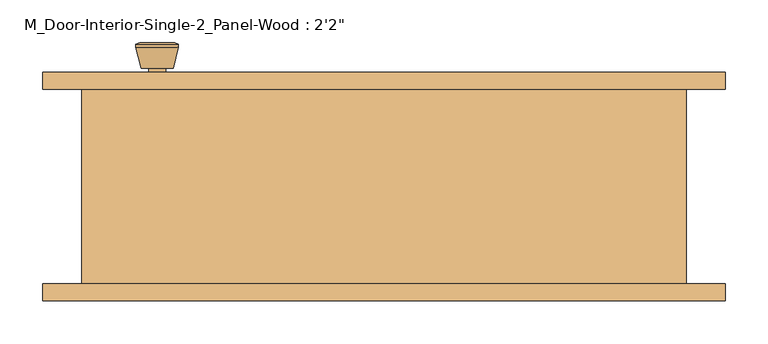
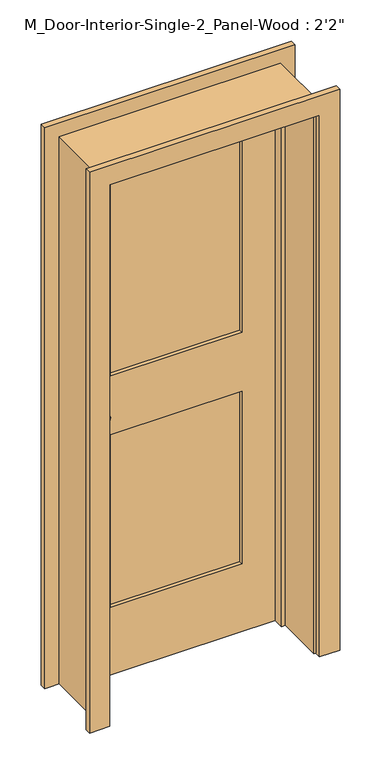
"""IFC4 building model written with IfcOpenShell, lengths in millimetres: door geometry."""

from ifc_helpers import new_model, si_unit, point, frame, frame_2d, origin, place, context, project, spatial, polyline, circle_curve, trimmed, segment, composite_curve, outline, extrude, faceted_brep, source, transform, mapped, element, save
from ifc_brep_helpers import plane_surface, cylinder_surface, revolved_surface, advanced_brep


def door_5f4ff63b(model_context):
    return source(origin(), model_context, "Body", "SolidModel", [
        advanced_brep(
        [(-266.7, 70.125, 914.4), (-256.7, 70.125, 914.4), (-276.7, 70.125, 914.4), (-246.2241324, 21.125, 914.4), (-266.7, 21.125, 914.4), (-287.1758676, 21.125, 914.4), (-241.7, 22.9528681, 914.4), (-291.7, 22.9528681, 914.4), (-241.7, 26.4165463, 914.4), (-291.7, 26.4165463, 914.4), (-248.063764, 51.125, 914.4), (-285.336236, 51.125, 914.4), (-256.7, 51.125, 914.4), (-276.7, 51.125, 914.4)],
        [
            (0, 1),
            (1, 2, circle_curve(frame((-266.7, 70.125, 914.4), z_axis=(0.0, 1.0, 0.0), x_axis=(-1.0, 0.0, 0.0)), 10.0)),
            (2, 0),
            (2, 1, circle_curve(frame((-266.7, 70.125, 914.4), z_axis=(0.0, 1.0, 0.0), x_axis=(-1.0, 0.0, 0.0)), 10.0)),
            (3, 4),
            (4, 5),
            (5, 3, circle_curve(frame((-266.7, 21.125, 914.4), z_axis=(0.0, -1.0, 0.0), x_axis=(-1.0, 0.0, 0.0)), 20.4758676)),
            (3, 5, circle_curve(frame((-266.7, 21.125, 914.4), z_axis=(0.0, -1.0, 0.0), x_axis=(-1.0, 0.0, 0.0)), 20.4758676)),
            (6, 3),
            (5, 7),
            (7, 6, circle_curve(frame((-266.7, 22.9528681, 914.4), z_axis=(0.0, -1.0, 0.0), x_axis=(-1.0, 0.0, 0.0)), 25.0)),
            (6, 7, circle_curve(frame((-266.7, 22.9528681, 914.4), z_axis=(0.0, -1.0, 0.0), x_axis=(-1.0, 0.0, 0.0)), 25.0)),
            (8, 6),
            (7, 9),
            (9, 8, circle_curve(frame((-266.7, 26.4165463, 914.4), z_axis=(0.0, -1.0, 0.0), x_axis=(-1.0, 0.0, 0.0)), 25.0)),
            (8, 9, circle_curve(frame((-266.7, 26.4165463, 914.4), z_axis=(0.0, -1.0, 0.0), x_axis=(-1.0, 0.0, 0.0)), 25.0)),
            (10, 8),
            (9, 11),
            (11, 10, circle_curve(frame((-266.7, 51.125, 914.4), z_axis=(0.0, -1.0, 0.0), x_axis=(-1.0, 0.0, 0.0)), 18.636236)),
            (10, 11, circle_curve(frame((-266.7, 51.125, 914.4), z_axis=(0.0, -1.0, 0.0), x_axis=(-1.0, 0.0, 0.0)), 18.636236)),
            (12, 10),
            (11, 13),
            (13, 12, circle_curve(frame((-266.7, 51.125, 914.4), z_axis=(0.0, -1.0, 0.0), x_axis=(-1.0, 0.0, 0.0)), 10.0)),
            (12, 13, circle_curve(frame((-266.7, 51.125, 914.4), z_axis=(0.0, -1.0, 0.0), x_axis=(-1.0, 0.0, 0.0)), 10.0)),
            (1, 12),
            (13, 2),
        ],
        [
            plane_surface(frame((-266.7, 70.125, 914.4), z_axis=(0.0, 1.0, 0.0), x_axis=(-1.0, 0.0, 0.0))),
            plane_surface(frame((-266.7, 21.125, 914.4), z_axis=(0.0, -1.0, 0.0), x_axis=(-1.0, 0.0, 0.0))),
            revolved_surface(polyline([(-287.1758676, 21.125, 914.4), (-291.7, 22.9528681, 914.4)]), (-266.7, 70.125, 914.4), (0.0, 1.0, 0.0)),
            cylinder_surface(frame((-266.7, 70.125, 914.4), z_axis=(0.0, 1.0, 0.0), x_axis=(-1.0, 0.0, 0.0)), 25.0),
            revolved_surface(polyline([(-291.7, 26.4165463, 914.4), (-285.336236, 51.125, 914.4)]), (-266.7, 70.125, 914.4), (0.0, 1.0, 0.0)),
            plane_surface(frame((-266.7, 51.125, 914.4), z_axis=(0.0, 1.0, 0.0), x_axis=(-1.0, 0.0, 0.0))),
            cylinder_surface(frame((-266.7, 70.125, 914.4), z_axis=(0.0, 1.0, 0.0), x_axis=(-1.0, 0.0, 0.0)), 10.0),
        ],
        [
            (0, [[1, 2, 3]]),
            (0, [[-3, 4, -1]]),
            (1, [[5, 6, 7]]),
            (1, [[-6, -5, 8]]),
            (2, [[9, -7, 10, 11]]),
            (2, [[-10, -8, -9, 12]]),
            (3, [[13, -11, 14, 15]]),
            (3, [[-14, -12, -13, 16]]),
            (4, [[17, -15, 18, 19]]),
            (4, [[-18, -16, -17, 20]]),
            (5, [[21, -19, 22, 23]]),
            (5, [[-22, -20, -21, 24]]),
            (6, [[25, -23, 26, -2]]),
            (6, [[-26, -24, -25, -4]]),
        ],
    ),
        extrude(outline(composite_curve([segment(trimmed(circle_curve(frame_2d((914.4, -266.7)), 30.0), [point((914.4, -296.7))], [point((914.4, -236.7))], False, "CARTESIAN"), True, "CONTINUOUS"), segment(trimmed(circle_curve(frame_2d((914.4, -266.7)), 30.0), [point((914.4, -236.7))], [point((914.4, -296.7))], False, "CARTESIAN"), True, "CONTINUOUS")], self_intersect=False)), frame((0.0, 70.125, 0.0), z_axis=(0.0, 1.0, 0.0), x_axis=(0.0, 0.0, 1.0)), (0.0, 0.0, 1.0), 6.0),
        advanced_brep(
        [(-266.7, 117.125, 914.4), (-276.7, 117.125, 914.4), (-256.7, 117.125, 914.4), (-246.2241324, 166.125, 914.4), (-287.1758676, 166.125, 914.4), (-266.7, 166.125, 914.4), (-241.7, 164.2971319, 914.4), (-291.7, 164.2971319, 914.4), (-241.7, 160.8334537, 914.4), (-291.7, 160.8334537, 914.4), (-248.063764, 136.125, 914.4), (-285.336236, 136.125, 914.4), (-256.7, 136.125, 914.4), (-276.7, 136.125, 914.4)],
        [
            (0, 1),
            (1, 2, circle_curve(frame((-266.7, 117.125, 914.4), z_axis=(0.0, -1.0, 0.0), x_axis=(-1.0, 0.0, 0.0)), 10.0)),
            (2, 0),
            (2, 1, circle_curve(frame((-266.7, 117.125, 914.4), z_axis=(0.0, -1.0, 0.0), x_axis=(-1.0, 0.0, 0.0)), 10.0)),
            (3, 4, circle_curve(frame((-266.7, 166.125, 914.4), z_axis=(0.0, 1.0, 0.0), x_axis=(-1.0, 0.0, 0.0)), 20.4758676)),
            (4, 5),
            (5, 3),
            (4, 3, circle_curve(frame((-266.7, 166.125, 914.4), z_axis=(0.0, 1.0, 0.0), x_axis=(-1.0, 0.0, 0.0)), 20.4758676)),
            (6, 7, circle_curve(frame((-266.7, 164.2971319, 914.4), z_axis=(0.0, 1.0, 0.0), x_axis=(-1.0, 0.0, 0.0)), 25.0)),
            (7, 4),
            (3, 6),
            (7, 6, circle_curve(frame((-266.7, 164.2971319, 914.4), z_axis=(0.0, 1.0, 0.0), x_axis=(-1.0, 0.0, 0.0)), 25.0)),
            (8, 9, circle_curve(frame((-266.7, 160.8334537, 914.4), z_axis=(0.0, 1.0, 0.0), x_axis=(-1.0, 0.0, 0.0)), 25.0)),
            (9, 7),
            (6, 8),
            (9, 8, circle_curve(frame((-266.7, 160.8334537, 914.4), z_axis=(0.0, 1.0, 0.0), x_axis=(-1.0, 0.0, 0.0)), 25.0)),
            (10, 11, circle_curve(frame((-266.7, 136.125, 914.4), z_axis=(0.0, 1.0, 0.0), x_axis=(-1.0, 0.0, 0.0)), 18.636236)),
            (11, 9),
            (8, 10),
            (11, 10, circle_curve(frame((-266.7, 136.125, 914.4), z_axis=(0.0, 1.0, 0.0), x_axis=(-1.0, 0.0, 0.0)), 18.636236)),
            (12, 13, circle_curve(frame((-266.7, 136.125, 914.4), z_axis=(0.0, 1.0, 0.0), x_axis=(-1.0, 0.0, 0.0)), 10.0)),
            (13, 11),
            (10, 12),
            (13, 12, circle_curve(frame((-266.7, 136.125, 914.4), z_axis=(0.0, 1.0, 0.0), x_axis=(-1.0, 0.0, 0.0)), 10.0)),
            (1, 13),
            (12, 2),
        ],
        [
            plane_surface(frame((-266.7, 117.125, 914.4), z_axis=(0.0, -1.0, 0.0), x_axis=(-1.0, 0.0, 0.0))),
            plane_surface(frame((-266.7, 166.125, 914.4), z_axis=(0.0, 1.0, 0.0), x_axis=(-1.0, 0.0, 0.0))),
            revolved_surface(polyline([(-287.1758676, 166.125, 914.4), (-291.7, 164.2971319, 914.4)]), (-266.7, 117.125, 914.4), (0.0, -1.0, 0.0)),
            cylinder_surface(frame((-266.7, 117.125, 914.4), z_axis=(0.0, -1.0, 0.0), x_axis=(-1.0, 0.0, 0.0)), 25.0),
            revolved_surface(polyline([(-291.7, 160.8334537, 914.4), (-285.336236, 136.125, 914.4)]), (-266.7, 117.125, 914.4), (0.0, -1.0, 0.0)),
            plane_surface(frame((-266.7, 136.125, 914.4), z_axis=(0.0, -1.0, 0.0), x_axis=(-1.0, 0.0, 0.0))),
            cylinder_surface(frame((-266.7, 117.125, 914.4), z_axis=(0.0, -1.0, 0.0), x_axis=(-1.0, 0.0, 0.0)), 10.0),
        ],
        [
            (0, [[1, 2, 3]]),
            (0, [[-3, 4, -1]]),
            (1, [[5, 6, 7]]),
            (1, [[8, -7, -6]]),
            (2, [[9, 10, -5, 11]]),
            (2, [[12, -11, -8, -10]]),
            (3, [[13, 14, -9, 15]]),
            (3, [[16, -15, -12, -14]]),
            (4, [[17, 18, -13, 19]]),
            (4, [[20, -19, -16, -18]]),
            (5, [[21, 22, -17, 23]]),
            (5, [[24, -23, -20, -22]]),
            (6, [[-2, 25, -21, 26]]),
            (6, [[-4, -26, -24, -25]]),
        ],
    ),
        extrude(outline(composite_curve([segment(trimmed(circle_curve(frame_2d((914.4, -266.7)), 30.0), [point((914.4, -296.7))], [point((914.4, -236.7))], False, "CARTESIAN"), True, "CONTINUOUS"), segment(trimmed(circle_curve(frame_2d((914.4, -266.7)), 30.0), [point((914.4, -236.7))], [point((914.4, -296.7))], False, "CARTESIAN"), True, "CONTINUOUS")], self_intersect=False)), frame((0.0, 111.125, 0.0), z_axis=(0.0, 1.0, 0.0), x_axis=(0.0, 0.0, 1.0)), (0.0, 0.0, 1.0), 6.0),
        faceted_brep([(355.2, 111.125, 0.0), (355.2, -117.475, 0.0), (330.2, -117.475, 0.0), (330.2, 41.2, 0.0), (317.5, 41.2, 0.0), (317.5, 76.125, 0.0), (330.2, 76.125, 0.0), (330.2, 111.125, 0.0), (355.2, 111.125, 1853.8), (355.2, -117.475, 1853.8), (-355.2, -117.475, 1853.8), (-355.2, -117.475, 0.0), (-330.2, -117.475, 0.0), (-330.2, -117.475, 1828.8), (330.2, -117.475, 1828.8), (330.2, 41.2, 1828.8), (-330.2, 41.2, 1828.8), (-330.2, 41.2, 0.0), (-317.5, 41.2, 0.0), (-317.5, 41.2, 1816.1), (317.5, 41.2, 1816.1), (317.5, 76.125, 1816.1), (-317.5, 76.125, 1816.1), (-317.5, 76.125, 0.0), (-330.2, 76.125, 0.0), (-330.2, 76.125, 1828.8), (330.2, 76.125, 1828.8), (330.2, 111.125, 1828.8), (-330.2, 111.125, 1828.8), (-330.2, 111.125, 0.0), (-355.2, 111.125, 0.0), (-355.2, 111.125, 1853.8)], [[[0, 1, 2, 3, 4, 5, 6, 7]], [[1, 0, 8, 9]], [[2, 1, 9, 10, 11, 12, 13, 14]], [[3, 2, 14, 15]], [[4, 3, 15, 16, 17, 18, 19, 20]], [[5, 4, 20, 21]], [[6, 5, 21, 22, 23, 24, 25, 26]], [[7, 6, 26, 27]], [[0, 7, 27, 28, 29, 30, 31, 8]], [[9, 8, 31, 10]], [[15, 14, 13, 16]], [[21, 20, 19, 22]], [[27, 26, 25, 28]], [[30, 29, 24, 23, 18, 17, 12, 11]], [[10, 31, 30, 11]], [[16, 13, 12, 17]], [[22, 19, 18, 23]], [[28, 25, 24, 29]]]),
        extrude(outline(polyline([(1828.8, -330.2), (0.0, -330.2), (0.0, 330.2), (1828.8, 330.2), (1828.8, -330.2)]), holes=[polyline([(1708.8, -210.2), (1708.8, 210.2), (1014.4, 210.2), (1014.4, -210.2), (1708.8, -210.2)]), polyline([(814.4, -210.2), (814.4, 210.2), (230.0, 210.2), (230.0, -210.2), (814.4, -210.2)])]), frame((0.0, 76.125, 0.0), z_axis=(0.0, 1.0, 0.0), x_axis=(0.0, 0.0, 1.0)), (0.0, 0.0, 1.0), 35.0),
        extrude(outline(polyline([(210.2, 87.7916667), (-210.2, 87.7916667), (-210.2, 99.4583333), (210.2, 99.4583333), (210.2, 87.7916667)])), frame((0.0, 0.0, 1014.4), z_axis=(0.0, 0.0, 1.0), x_axis=(1.0, 0.0, 0.0)), (0.0, 0.0, 1.0), 694.4),
        extrude(outline(polyline([(210.2, 87.7916667), (-210.2, 87.7916667), (-210.2, 99.4583333), (210.2, 99.4583333), (210.2, 87.7916667)])), frame((0.0, 0.0, 230.0), z_axis=(0.0, 0.0, 1.0), x_axis=(1.0, 0.0, 0.0)), (0.0, 0.0, 1.0), 584.4),
        extrude(outline(polyline([(0.0, 336.55), (0.0, 401.55), (1900.15, 401.55), (1900.15, -401.55), (0.0, -401.55), (0.0, -336.55), (1835.15, -336.55), (1835.15, 336.55), (0.0, 336.55)])), frame((0.0, 111.125, 0.0), z_axis=(0.0, 1.0, 0.0), x_axis=(0.0, 0.0, 1.0)), (0.0, 0.0, 1.0), 20.0),
        extrude(outline(polyline([(0.0, 336.55), (0.0, 401.55), (1900.15, 401.55), (1900.15, -401.55), (0.0, -401.55), (0.0, -336.55), (1835.15, -336.55), (1835.15, 336.55), (0.0, 336.55)])), frame((0.0, -137.475, 0.0), z_axis=(0.0, 1.0, 0.0), x_axis=(0.0, 0.0, 1.0)), (0.0, 0.0, 1.0), 20.0),
    ])


if __name__ == "__main__":
    model = new_model("IFC4")
    model_context = context("Model", 3, world=origin())
    ifc_project = project(units=[si_unit("LENGTHUNIT", "METRE", prefix="MILLI")], contexts=[model_context])
    site = spatial("IfcSite", under=ifc_project)
    building = spatial("IfcBuilding", under=site)
    placement = place(None, origin())
    door_shape = door_5f4ff63b(model_context)
    element("IfcDoor", 1, ObjectType="M_Door-Interior-Single-2_Panel-Wood : 2'2\"", at=placement, inside=building, context=model_context, shape_type="MappedRepresentation", body=[
        mapped(door_shape, transform((0.0, 0.0, 0.0), x_axis=(1.0, 0.0, 0.0), y_axis=(0.0, 1.0, 0.0), z_axis=(0.0, 0.0, 1.0))),
    ])
    save(model, "model.ifc")

# Revit data of these elements
# Type "M_Door-Interior-Single-2_Panel-Wood : 2'2\""
#   Type Mark = "11"
#   Assembly Code = "C1020300"
#   Analytic Construction = "Wooden"
#   Top Rail = 0' - 4.72441"
#   Thickness = 0' - 1.37795"
#   Thermal Resistance (R) = 2.5876 (h·ft²·°F)/BTU
#   Swing Angle [instance default] = 90.00°
#   Stiles = 0' - 4.72441"
#   Rough Width = 2' - 3.9685"
#   Rough Height = 6' - 0.98425"
#   Lock Rail = 0' - 7.87402"
#   Height = 6' - 0"
#   Width = 2' - 2"
#   Heat Transfer Coefficient (U) = 0.3865 BTU/(h·ft²·°F)
#   Bottom Rail = 0' - 9.05512"
#   Trim Material = Cherry
#   Panel Material = Cherry
#   Frame Material = Cherry
#   Door Handle Material = Aluminum
#   Visual Light Transmittance = 0
#   Solar Heat Gain Coefficient = 0
#   Wall Closure = (empty or 0)
#   Function = (empty or 0)
# Element 1 (IfcDoor, "M_Door-Interior-Single-2_Panel-Wood : 2'2\"")
#   Materials on its faces: "Cherry", "Aluminum"
# Materials
#   "Cherry": class "Wood", colour RGB 226 177 128, transparency 0, Description = "Prunus Serotina", Cost = 0
#   "Aluminum": class "Metal", colour RGB 247 247 247, transparency 0, Description = "Aluminum 6061", Cost = 0
